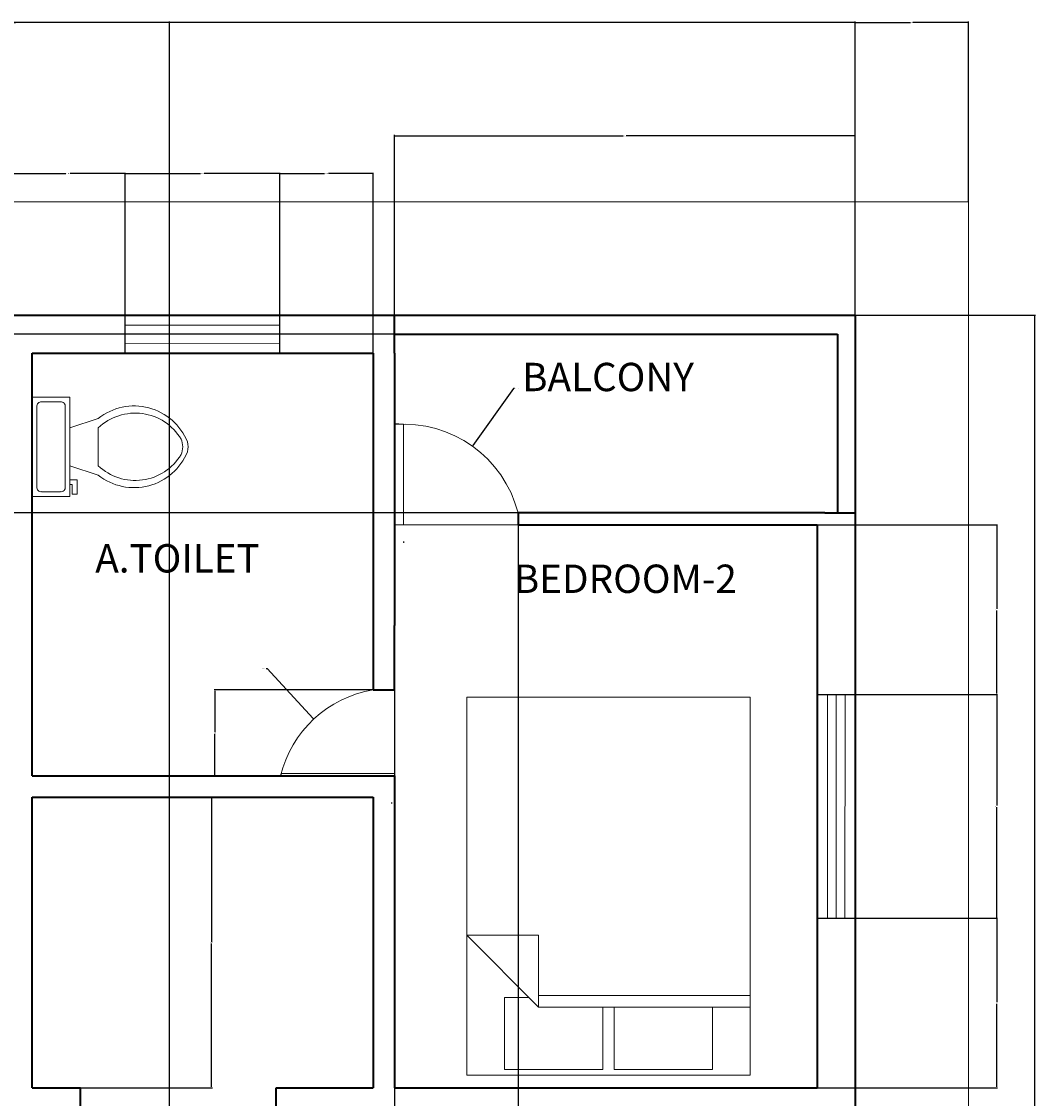
# Model space of a CAD drawing. Units: inches. Extents: x 4700 to 5209, y 8078 to 8754.
# Tile 5 of 5: x 4970 to 5185, y 8526 to 8754. Entities that reach past the tile are written whole.
import ezdxf

# ---------------------------------------------------------------- set-up
doc = ezdxf.new("R2010")
doc.units = ezdxf.units.IN
for name, color, linetype, lineweight in [('A-ANNO-DIMS', 2, 'Continuous', 18), ('A-AREA-IDEN', 7, 'Continuous', 18), ('A-DOOR', 3, 'Continuous', 18), ('A-FLOR-FIXT', 9, 'Continuous', 18), ('A-FURN', 8, 'Continuous', 18), ('A-GLAZ', 4, 'Continuous', 18), ('A-WALL', 7, 'Continuous', 35), ('C-PROP', 8, 'Continuous', 18)]:
    doc.layers.add(name, color=color, linetype=linetype, lineweight=lineweight)
doc.styles.get("Standard").update_dxf_attribs({"font": 'arial.ttf'})
doc.dimstyles.get("Standard").update_dxf_attribs({"dimtxt": 0.18, "dimasz": 0.18, "dimexe": 0.18, "dimexo": 0.0625, "dimgap": 0.09, "dimtad": 0, "dimtih": 1, "dimtoh": 1, "dimdec": 4, "dimzin": 0, "dimdsep": 46, "dimtxsty": 'Standard', "dimcen": 0.09, "dimadec": 0, "dimazin": 0, "dimtfac": 1, "dimtdec": 4, "dimtofl": 0, "dimtmove": 0, "dimatfit": 3, "dimfxl": 1, "dimtolj": 1, "dimtzin": 0, "dimarcsym": 0})

# ---------------------------------------------------------------- blocks, each defined once
blk = doc.blocks.new('Bed - Queen')
for p, q in [((0, -80.00003), (0, 0)), ((0, 0), (59.99999, 0)), ((59.99999, 0), (59.99999, -80.00003)), ((7.99999, -1.2), (28.79998, -1.2)), ((7.99999, -14.4), (7.99999, -1.2)), ((28.79998, -1.2), (28.79998, -14.4)), ((31.19999, -1.2), (51.99999, -1.2)), ((31.19999, -14.4), (31.19999, -1.2)), ((51.99999, -1.2), (51.99999, -16.4)), ((0, -14.4), (44.8, -14.4)), ((59.99999, -29.6), (44.8, -14.4)), ((44.8, -14.4), (44.8, -29.6)), ((44.8, -16.8), (0, -16.8)), ((51.99999, -16.4), (46.79936, -16.4)), ((44.8, -29.6), (59.99999, -29.6)), ((59.99999, -80.00003), (0, -80.00003))]:
    blk.add_line(p, q)
blk = doc.blocks.new('Toilet - top')
for p, q in [((9.5, -6), (9.5, -2)), ((-10, -8.5), (-8, -8.5)), ((-10, -9.5), (-10, -8.5)), ((-8, -8.5), (-8, -8)), ((-7, -8), (-7, -9.5)), ((-4, -8), (-6, -14)), ((4, -8), (6, -14)), ((-7, -9.5), (-10, -9.5)), ((4, -14), (-4, -14))]:
    blk.add_line(p, q)
blk.add_lwpolyline([(10.5, -8), (10.5, 0), (-10.5, 0), (-10.5, -8)], close=True)
for points in [[(-9.5, -2), (-9.5, -6)], [(8.5, -1), (-8.5, -1)], [(-8.5, -7), (8.5, -7)]]:
    blk.add_lwpolyline(points)
for centre, radius, start, end in [((-8.62, -1.88), 0.884, 81.8699, 188.1301), ((8.62, -1.88), 0.884, 351.8699, 98.1301), ((-8.62, -6.12), 0.884, 171.8699, 278.1301), ((8.62, -6.12), 0.884, 261.8699, 8.1301), ((3.52, -21.58), 12.17, 141.4691, 247.9714), ((4.2, -21.82), 11.33, 136.3677, 238.9468), ((-3.52, -21.58), 12.17, 292.0284, 38.5307), ((-4.2, -21.82), 11.33, 301.053, 43.6321), ((0, -27.88), 4, 245.7318, 294.2682), ((0, -29), 4, 254.8605, 285.1395)]:
    blk.add_arc(centre, radius, start, end)
blk = doc.blocks.new('*D16')
at = {"layer": 'A-ANNO-DIMS', "color": 0, "lineweight": -2, "transparency": 16777216}
for p, q in [((4762.78, 8691.81), (4762.78, 8753.93)), ((4762.96, 8753.75), (4954.49, 8753.75)), ((5146.6, 8753.75), (4955.07, 8753.75)), ((5146.78, 8691.81), (5146.78, 8753.93))]:
    blk.add_line(p, q, dxfattribs=at)
at = {"layer": 'A-ANNO-DIMS', "color": 0, "transparency": 16777216}
for points in [[(4762.96, 8753.78), (4762.96, 8753.72), (4762.78, 8753.75)], [(5146.6, 8753.78), (5146.6, 8753.72), (5146.78, 8753.75)]]:
    blk.add_solid(points, dxfattribs=at)
at = {"layer": 'Defpoints', "color": 0, "transparency": 16777216}
for p in [(5146.78, 8753.75), (4762.78, 8691.75), (5146.78, 8691.75)]:
    blk.add_point(p, dxfattribs=at)
at = {"layer": 'A-ANNO-DIMS', "color": 0, "transparency": 16777216, "insert": (4954.78, 8753.75), "char_height": 0.18, "attachment_point": 5}
blk.add_mtext('\\A1;384', dxfattribs=at)
blk = doc.blocks.new('*D17')
at = {"layer": 'A-ANNO-DIMS', "color": 0, "lineweight": -2, "transparency": 16777216}
for p, q in [((5146.84, 8691.75), (5184.96, 8691.75)), ((5184.78, 8691.57), (5184.78, 8403.93)), ((5184.78, 8115.93), (5184.78, 8403.57)), ((5146.84, 8115.75), (5184.96, 8115.75))]:
    blk.add_line(p, q, dxfattribs=at)
at = {"layer": 'A-ANNO-DIMS', "color": 0, "transparency": 16777216}
for points in [[(5184.75, 8691.57), (5184.81, 8691.57), (5184.78, 8691.75)], [(5184.75, 8115.93), (5184.81, 8115.93), (5184.78, 8115.75)]]:
    blk.add_solid(points, dxfattribs=at)
at = {"layer": 'Defpoints', "color": 0, "transparency": 16777216}
for p in [(5146.78, 8691.75), (5146.78, 8115.75), (5184.78, 8115.75)]:
    blk.add_point(p, dxfattribs=at)
at = {"layer": 'A-ANNO-DIMS', "color": 0, "transparency": 16777216, "insert": (5184.78, 8403.75), "char_height": 0.18, "attachment_point": 5}
blk.add_mtext('\\A1;576', dxfattribs=at)
blk = doc.blocks.new('*D24')
at = {"layer": 'A-ANNO-DIMS', "color": 0, "lineweight": -2, "transparency": 16777216}
for p, q in [((4968.07, 8683.81), (4968.07, 8721.93)), ((4968.25, 8721.75), (4979.68, 8721.75)), ((4992.05, 8721.75), (4980.61, 8721.75)), ((4992.23, 8683.81), (4992.23, 8721.93))]:
    blk.add_line(p, q, dxfattribs=at)
at = {"layer": 'A-ANNO-DIMS', "color": 0, "transparency": 16777216}
for points in [[(4968.25, 8721.78), (4968.25, 8721.72), (4968.07, 8721.75)], [(4992.05, 8721.78), (4992.05, 8721.72), (4992.23, 8721.75)]]:
    blk.add_solid(points, dxfattribs=at)
at = {"layer": 'Defpoints', "color": 0, "transparency": 16777216}
for p in [(4992.23, 8721.75), (4968.07, 8683.75), (4992.23, 8683.75)]:
    blk.add_point(p, dxfattribs=at)
at = {"layer": 'A-ANNO-DIMS', "color": 0, "transparency": 16777216, "insert": (4980.15, 8721.75), "char_height": 0.18, "attachment_point": 5}
blk.add_mtext('\\A1;24.153', dxfattribs=at)
blk = doc.blocks.new('*D25')
at = {"layer": 'A-ANNO-DIMS', "color": 0, "lineweight": -2, "transparency": 16777216}
for p, q in [((4992.23, 8683.81), (4992.23, 8721.93)), ((4992.41, 8721.75), (5008.22, 8721.75)), ((5024.82, 8721.75), (5009.01, 8721.75)), ((5025, 8683.81), (5025, 8721.93))]:
    blk.add_line(p, q, dxfattribs=at)
at = {"layer": 'A-ANNO-DIMS', "color": 0, "transparency": 16777216}
for points in [[(4992.41, 8721.78), (4992.41, 8721.72), (4992.23, 8721.75)], [(5024.82, 8721.78), (5024.82, 8721.72), (5025, 8721.75)]]:
    blk.add_solid(points, dxfattribs=at)
at = {"layer": 'Defpoints', "color": 0, "transparency": 16777216}
for p in [(5025, 8721.75), (4992.23, 8683.75), (5025, 8683.75)]:
    blk.add_point(p, dxfattribs=at)
at = {"layer": 'A-ANNO-DIMS', "color": 0, "transparency": 16777216, "insert": (5008.61, 8721.75), "char_height": 0.18, "attachment_point": 5}
blk.add_mtext('\\A1;32.77', dxfattribs=at)
blk = doc.blocks.new('*D26')
at = {"layer": 'A-ANNO-DIMS', "color": 0, "lineweight": -2, "transparency": 16777216}
for p, q in [((5025, 8683.81), (5025, 8721.93)), ((5025.18, 8721.75), (5034.43, 8721.75)), ((5044.6, 8721.75), (5035.34, 8721.75)), ((5044.78, 8683.81), (5044.78, 8721.93))]:
    blk.add_line(p, q, dxfattribs=at)
at = {"layer": 'A-ANNO-DIMS', "color": 0, "transparency": 16777216}
for points in [[(5025.18, 8721.78), (5025.18, 8721.72), (5025, 8721.75)], [(5044.6, 8721.78), (5044.6, 8721.72), (5044.78, 8721.75)]]:
    blk.add_solid(points, dxfattribs=at)
at = {"layer": 'Defpoints', "color": 0, "transparency": 16777216}
for p in [(5044.78, 8721.75), (5025, 8683.75), (5044.78, 8683.75)]:
    blk.add_point(p, dxfattribs=at)
at = {"layer": 'A-ANNO-DIMS', "color": 0, "transparency": 16777216, "insert": (5034.89, 8721.75), "char_height": 0.18, "attachment_point": 5}
blk.add_mtext('\\A1;19.782', dxfattribs=at)
blk = doc.blocks.new('*D27')
at = {"layer": 'A-ANNO-DIMS', "color": 0, "lineweight": -2, "transparency": 16777216}
for p, q in [((5049.28, 8691.81), (5049.28, 8729.93)), ((5049.46, 8729.75), (5097.71, 8729.75)), ((5146.6, 8729.75), (5098.35, 8729.75)), ((5146.78, 8691.81), (5146.78, 8729.93))]:
    blk.add_line(p, q, dxfattribs=at)
at = {"layer": 'A-ANNO-DIMS', "color": 0, "transparency": 16777216}
for points in [[(5049.46, 8729.78), (5049.46, 8729.72), (5049.28, 8729.75)], [(5146.6, 8729.78), (5146.6, 8729.72), (5146.78, 8729.75)]]:
    blk.add_solid(points, dxfattribs=at)
at = {"layer": 'Defpoints', "color": 0, "transparency": 16777216}
for p in [(5146.78, 8729.75), (5049.28, 8691.75), (5146.78, 8691.75)]:
    blk.add_point(p, dxfattribs=at)
at = {"layer": 'A-ANNO-DIMS', "color": 0, "transparency": 16777216, "insert": (5098.03, 8729.75), "char_height": 0.18, "attachment_point": 5}
blk.add_mtext('\\A1;97.5', dxfattribs=at)
blk = doc.blocks.new('*D44')
at = {"layer": 'A-ANNO-DIMS', "color": 0, "lineweight": -2, "transparency": 16777216}
for p, q in [((5138.84, 8564.15), (5176.96, 8564.15)), ((5176.78, 8563.97), (5176.78, 8546.38)), ((5176.78, 8528.43), (5176.78, 8546.02)), ((5138.84, 8528.25), (5176.96, 8528.25))]:
    blk.add_line(p, q, dxfattribs=at)
at = {"layer": 'A-ANNO-DIMS', "color": 0, "transparency": 16777216}
for points in [[(5176.75, 8563.97), (5176.81, 8563.97), (5176.78, 8564.15)], [(5176.75, 8528.43), (5176.81, 8528.43), (5176.78, 8528.25)]]:
    blk.add_solid(points, dxfattribs=at)
at = {"layer": 'Defpoints', "color": 0, "transparency": 16777216}
for p in [(5138.78, 8564.15), (5138.78, 8528.25), (5176.78, 8528.25)]:
    blk.add_point(p, dxfattribs=at)
at = {"layer": 'A-ANNO-DIMS', "color": 0, "transparency": 16777216, "insert": (5176.78, 8546.2), "char_height": 0.18, "attachment_point": 5}
blk.add_mtext('\\A1;35.9', dxfattribs=at)
blk = doc.blocks.new('*D45')
at = {"layer": 'A-ANNO-DIMS', "color": 0, "lineweight": -2, "transparency": 16777216}
for p, q in [((5138.84, 8611.51), (5176.96, 8611.51)), ((5176.78, 8611.33), (5176.78, 8588.01)), ((5176.78, 8564.33), (5176.78, 8587.65)), ((5138.84, 8564.15), (5176.96, 8564.15))]:
    blk.add_line(p, q, dxfattribs=at)
at = {"layer": 'A-ANNO-DIMS', "color": 0, "transparency": 16777216}
for points in [[(5176.75, 8611.33), (5176.81, 8611.33), (5176.78, 8611.51)], [(5176.75, 8564.33), (5176.81, 8564.33), (5176.78, 8564.15)]]:
    blk.add_solid(points, dxfattribs=at)
at = {"layer": 'Defpoints', "color": 0, "transparency": 16777216}
for p in [(5138.78, 8611.51), (5138.78, 8564.15), (5176.78, 8564.15)]:
    blk.add_point(p, dxfattribs=at)
at = {"layer": 'A-ANNO-DIMS', "color": 0, "transparency": 16777216, "insert": (5176.78, 8587.83), "char_height": 0.18, "attachment_point": 5}
blk.add_mtext('\\A1;47.36', dxfattribs=at)
blk = doc.blocks.new('*D46')
at = {"layer": 'A-ANNO-DIMS', "color": 0, "lineweight": -2, "transparency": 16777216}
for p, q in [((5138.84, 8647.41), (5176.96, 8647.41)), ((5176.78, 8647.23), (5176.78, 8629.64)), ((5176.78, 8611.69), (5176.78, 8629.28)), ((5138.84, 8611.51), (5176.96, 8611.51))]:
    blk.add_line(p, q, dxfattribs=at)
at = {"layer": 'A-ANNO-DIMS', "color": 0, "transparency": 16777216}
for points in [[(5176.75, 8647.23), (5176.81, 8647.23), (5176.78, 8647.41)], [(5176.75, 8611.69), (5176.81, 8611.69), (5176.78, 8611.51)]]:
    blk.add_solid(points, dxfattribs=at)
at = {"layer": 'Defpoints', "color": 0, "transparency": 16777216}
for p in [(5138.78, 8647.41), (5138.78, 8611.51), (5176.78, 8611.51)]:
    blk.add_point(p, dxfattribs=at)
at = {"layer": 'A-ANNO-DIMS', "color": 0, "transparency": 16777216, "insert": (5176.78, 8629.46), "char_height": 0.18, "attachment_point": 5}
blk.add_mtext('\\A1;35.89', dxfattribs=at)
blk = doc.blocks.new('*D47')
at = {"layer": 'A-ANNO-DIMS', "color": 0, "lineweight": -2, "transparency": 16777216}
for p, q in [((5142.99, 8687.75), (4700.6, 8687.75)), ((4700.78, 8687.57), (4700.78, 8669.03)), ((4700.78, 8650.12), (4700.78, 8668.66)), ((5142.99, 8649.94), (4700.6, 8649.94))]:
    blk.add_line(p, q, dxfattribs=at)
at = {"layer": 'A-ANNO-DIMS', "color": 0, "transparency": 16777216}
for points in [[(4700.75, 8687.57), (4700.81, 8687.57), (4700.78, 8687.75)], [(4700.75, 8650.12), (4700.81, 8650.12), (4700.78, 8649.94)]]:
    blk.add_solid(points, dxfattribs=at)
at = {"layer": 'Defpoints', "color": 0, "transparency": 16777216}
for p in [(5143.05, 8687.75), (4700.78, 8649.94), (5143.05, 8649.94)]:
    blk.add_point(p, dxfattribs=at)
at = {"layer": 'A-ANNO-DIMS', "color": 0, "transparency": 16777216, "insert": (4700.78, 8668.84), "char_height": 0.18, "attachment_point": 5}
blk.add_mtext('\\A1;37.814', dxfattribs=at)
blk = doc.blocks.new('*D55')
at = {"layer": 'A-ANNO-DIMS', "color": 0, "lineweight": -2, "transparency": 16777216}
for p, q in [((4937.15, 8207.81), (4937.15, 8753.93)), ((4937.33, 8753.75), (4969.02, 8753.75)), ((5001.49, 8753.75), (4969.8, 8753.75)), ((5001.67, 8207.81), (5001.67, 8753.93))]:
    blk.add_line(p, q, dxfattribs=at)
at = {"layer": 'A-ANNO-DIMS', "color": 0, "transparency": 16777216}
for points in [[(4937.33, 8753.78), (4937.33, 8753.72), (4937.15, 8753.75)], [(5001.49, 8753.78), (5001.49, 8753.72), (5001.67, 8753.75)]]:
    blk.add_solid(points, dxfattribs=at)
at = {"layer": 'Defpoints', "color": 0, "transparency": 16777216}
for p in [(5001.67, 8753.75), (4937.15, 8207.75), (5001.67, 8207.75)]:
    blk.add_point(p, dxfattribs=at)
at = {"layer": 'A-ANNO-DIMS', "color": 0, "transparency": 16777216, "insert": (4969.41, 8753.75), "char_height": 0.18, "attachment_point": 5}
blk.add_mtext('\\A1;64.53', dxfattribs=at)
blk = doc.blocks.new('*D59')
at = {"layer": 'A-ANNO-DIMS', "color": 0, "lineweight": -2, "transparency": 16777216}
for p, q in [((4972.64, 8589.75), (5010.75, 8589.75)), ((5010.57, 8589.57), (5010.57, 8559.18)), ((5010.57, 8528.43), (5010.57, 8558.82)), ((4972.64, 8528.25), (5010.75, 8528.25))]:
    blk.add_line(p, q, dxfattribs=at)
at = {"layer": 'A-ANNO-DIMS', "color": 0, "transparency": 16777216}
for points in [[(5010.54, 8589.57), (5010.6, 8589.57), (5010.57, 8589.75)], [(5010.54, 8528.43), (5010.6, 8528.43), (5010.57, 8528.25)]]:
    blk.add_solid(points, dxfattribs=at)
at = {"layer": 'Defpoints', "color": 0, "transparency": 16777216}
for p in [(4972.57, 8589.75), (4972.57, 8528.25), (5010.57, 8528.25)]:
    blk.add_point(p, dxfattribs=at)
at = {"layer": 'A-ANNO-DIMS', "color": 0, "transparency": 16777216, "insert": (5010.57, 8559), "char_height": 0.18, "attachment_point": 5}
blk.add_mtext('\\A1;61.5', dxfattribs=at)
blk = doc.blocks.new('*D68')
at = {"layer": 'A-ANNO-DIMS', "color": 0, "lineweight": -2, "transparency": 16777216}
for p, q in [((5049.22, 8612.47), (5011.1, 8612.47)), ((5011.28, 8612.29), (5011.28, 8603.54)), ((5011.28, 8594.43), (5011.28, 8603.18)), ((5049.22, 8594.25), (5011.1, 8594.25))]:
    blk.add_line(p, q, dxfattribs=at)
at = {"layer": 'A-ANNO-DIMS', "color": 0, "transparency": 16777216}
for points in [[(5011.25, 8612.29), (5011.31, 8612.29), (5011.28, 8612.47)], [(5011.25, 8594.43), (5011.31, 8594.43), (5011.28, 8594.25)]]:
    blk.add_solid(points, dxfattribs=at)
at = {"layer": 'Defpoints', "color": 0, "transparency": 16777216}
for p in [(5011.28, 8612.47), (5049.28, 8612.47), (5049.28, 8594.25)]:
    blk.add_point(p, dxfattribs=at)
at = {"layer": 'A-ANNO-DIMS', "color": 0, "transparency": 16777216, "insert": (5011.28, 8603.36), "char_height": 0.18, "attachment_point": 5}
blk.add_mtext('\\A1;18.215', dxfattribs=at)
blk = doc.blocks.new('*D71')
at = {"layer": 'A-ANNO-DIMS', "color": 0, "lineweight": -2, "transparency": 16777216}
for p, q in [((5049.28, 8647.34), (5049.28, 8077.57)), ((5075.44, 8647.34), (5075.44, 8077.57)), ((5049.46, 8077.75), (5061.97, 8077.75)), ((5075.26, 8077.75), (5062.76, 8077.75))]:
    blk.add_line(p, q, dxfattribs=at)
at = {"layer": 'A-ANNO-DIMS', "color": 0, "transparency": 16777216}
for points in [[(5049.46, 8077.78), (5049.46, 8077.72), (5049.28, 8077.75)], [(5075.26, 8077.78), (5075.26, 8077.72), (5075.44, 8077.75)]]:
    blk.add_solid(points, dxfattribs=at)
at = {"layer": 'Defpoints', "color": 0, "transparency": 16777216}
for p in [(5049.28, 8647.41), (5075.44, 8647.41), (5075.44, 8077.75)]:
    blk.add_point(p, dxfattribs=at)
at = {"layer": 'A-ANNO-DIMS', "color": 0, "transparency": 16777216, "insert": (5062.36, 8077.75), "char_height": 0.18, "attachment_point": 5}
blk.add_mtext('\\A1;26.16', dxfattribs=at)
blk = doc.blocks.new('*D73')
at = {"layer": 'A-ANNO-DIMS', "color": 0, "lineweight": -2, "transparency": 16777216}
for p, q in [((5146.78, 8691.81), (5146.78, 8753.93)), ((5146.96, 8753.75), (5158.56, 8753.75)), ((5170.6, 8753.75), (5159, 8753.75)), ((5170.78, 8715.81), (5170.78, 8753.93))]:
    blk.add_line(p, q, dxfattribs=at)
at = {"layer": 'A-ANNO-DIMS', "color": 0, "transparency": 16777216}
for points in [[(5146.96, 8753.78), (5146.96, 8753.72), (5146.78, 8753.75)], [(5170.6, 8753.78), (5170.6, 8753.72), (5170.78, 8753.75)]]:
    blk.add_solid(points, dxfattribs=at)
at = {"layer": 'Defpoints', "color": 0, "transparency": 16777216}
for p in [(5170.78, 8753.75), (5170.78, 8715.75), (5146.78, 8691.75)]:
    blk.add_point(p, dxfattribs=at)
at = {"layer": 'A-ANNO-DIMS', "color": 0, "transparency": 16777216, "insert": (5158.78, 8753.75), "char_height": 0.18, "attachment_point": 5}
blk.add_mtext('\\A1;24', dxfattribs=at)
blk = doc.blocks.new('*D83')
at = {"layer": 'A-ANNO-DIMS', "color": 0, "lineweight": -2, "transparency": 16777216}
for p, q in [((5074.48, 8676.24), (5065.88, 8664.21)), ((5074.66, 8676.24), (5074.48, 8676.24)), ((5051.17, 8643.76), (5051.35, 8643.76)), ((5051.26, 8643.67), (5051.26, 8643.85))]:
    blk.add_line(p, q, dxfattribs=at)
at = {"layer": 'A-ANNO-DIMS', "color": 0, "transparency": 16777216}
blk.add_solid([(5065.85, 8664.23), (5065.9, 8664.19), (5065.77, 8664.06)], dxfattribs=at)
at = {"layer": 'Defpoints', "color": 0, "transparency": 16777216}
for p in [(5065.77, 8664.06), (5051.26, 8643.76)]:
    blk.add_point(p, dxfattribs=at)
at = {"layer": 'A-ANNO-DIMS', "color": 0, "transparency": 16777216, "insert": (5075.21, 8676.24), "char_height": 0.18, "attachment_point": 5}
blk.add_mtext('\\A1;R24.955', dxfattribs=at)
blk = doc.blocks.new('*D84')
at = {"layer": 'A-ANNO-DIMS', "color": 0, "lineweight": -2, "transparency": 16777216}
for p, q in [((5022.15, 8616.98), (5022.33, 8616.98)), ((5022.33, 8616.98), (5032.09, 8606.45)), ((5048.6, 8588.55), (5048.78, 8588.55)), ((5048.69, 8588.46), (5048.69, 8588.64))]:
    blk.add_line(p, q, dxfattribs=at)
at = {"layer": 'A-ANNO-DIMS', "color": 0, "transparency": 16777216}
blk.add_solid([(5032.11, 8606.47), (5032.07, 8606.43), (5032.21, 8606.32)], dxfattribs=at)
at = {"layer": 'Defpoints', "color": 0, "transparency": 16777216}
for p in [(5032.21, 8606.32), (5048.69, 8588.55)]:
    blk.add_point(p, dxfattribs=at)
at = {"layer": 'A-ANNO-DIMS', "color": 0, "transparency": 16777216, "insert": (5021.67, 8616.98), "char_height": 0.18, "attachment_point": 5}
blk.add_mtext('\\A1;R24.23', dxfattribs=at)

msp = doc.modelspace()

# ---------------------------------------------------------------- linework, layer by layer
at = {"layer": 'A-DOOR'}
for p, q in [((5051.21, 8668.7155), (5049.2803, 8668.8641)), ((5051.21, 8647.4059), (5051.21, 8668.7155)), ((5049.2803, 8647.4059), (5051.21, 8647.4059)), ((5051.21, 8647.4059), (5075.4408, 8647.4059)), ((5049.2803, 8612.4657), (5049.2803, 8594.2503)), ((5049.2803, 8594.7861), (5025.2753, 8594.7861)), ((5025.2753, 8594.7861), (5025.2753, 8594.2503)), ((5049.2803, 8594.2503), (5049.2803, 8594.7861))]:
    msp.add_line(p, q, dxfattribs=at)
for centre, radius, start, end in [((5051.2623, 8643.7608), 24.9547, 14.328007, 94.555505), ((5048.6891, 8588.5541), 24.229, 99.28391, 166.402517)]:
    msp.add_arc(centre, radius, start, end, dxfattribs=at)
at = {"layer": 'A-GLAZ'}
for p, q in [((4992.2261, 8689.6376), (5024.9979, 8689.6376)), ((4992.2261, 8687.7503), (5024.9979, 8687.7503)), ((4992.2261, 8685.876), (5024.9979, 8685.8133)), ((5140.9607, 8611.5136), (5140.9607, 8564.1518)), ((5142.7803, 8611.5136), (5142.7803, 8564.1518)), ((5144.7087, 8611.5136), (5144.6194, 8564.1518))]:
    msp.add_line(p, q, dxfattribs=at)
for points in [[(4992.2261, 8691.7503), (5024.9979, 8691.7503), (5024.9979, 8683.7503), (4992.2261, 8683.7503)], [(5138.7803, 8611.5136), (5146.7803, 8611.5136), (5146.7803, 8564.1518), (5138.7803, 8564.1518)]]:
    msp.add_lwpolyline(points, close=True, dxfattribs=at)
at = {"layer": 'A-WALL'}
for p, q in [((4762.7803, 8691.7503), (5146.7803, 8691.7503)), ((5049.2803, 8683.7503), (5049.2803, 8691.7503)), ((5146.7803, 8691.7503), (5146.7803, 8199.7503)), ((5049.2803, 8687.7503), (5143.0547, 8687.7503)), ((5143.0547, 8687.7503), (5143.0547, 8649.9364)), ((4972.5733, 8683.7503), (5044.7803, 8683.7503)), ((4972.5733, 8594.2503), (4972.5733, 8683.7503)), ((5044.7803, 8683.7503), (5044.7803, 8626.0977)), ((5049.2803, 8683.7503), (5049.2803, 8626.0977)), ((5140.3862, 8649.9364), (5075.4408, 8649.9364)), ((5075.4408, 8649.9364), (5075.4408, 8647.4059)), ((5140.3862, 8649.9364), (5146.7803, 8649.9364)), ((5075.4408, 8647.4059), (5138.7803, 8647.4059)), ((5138.7803, 8647.4059), (5138.7803, 8528.2503)), ((5044.7803, 8626.0977), (5044.7803, 8612.4657)), ((5049.2803, 8612.4657), (5049.2803, 8626.0977)), ((5044.7803, 8612.4657), (5049.2803, 8612.4657)), ((4972.5733, 8594.2503), (5044.7803, 8594.2503)), ((5044.7803, 8594.2503), (5049.2803, 8594.2503)), ((5049.2803, 8594.2503), (5049.2803, 8528.2503)), ((4972.5733, 8528.2503), (4972.5733, 8589.7503)), ((4972.5733, 8589.7503), (5044.7803, 8589.7503)), ((5044.7803, 8589.7503), (5044.7803, 8528.2503)), ((4972.5733, 8528.2503), (4982.778, 8528.2503)), ((4982.778, 8523.7503), (4982.778, 8528.2503)), ((5024.2192, 8523.7503), (5024.2192, 8528.2503)), ((5024.2192, 8528.2503), (5044.7803, 8528.2503)), ((5049.2803, 8528.2503), (5138.7803, 8528.2503))]:
    msp.add_line(p, q, dxfattribs=at)
at = {"layer": 'C-PROP'}
for p, q in [((4738.7803, 8715.7503), (5170.7803, 8715.7503)), ((5170.7803, 8715.7503), (5170.7803, 8115.7503))]:
    msp.add_line(p, q, dxfattribs=at)

# ---------------------------------------------------------------- block references
at = {"layer": 'A-FLOR-FIXT', "rotation": 90}
msp.add_blockref('Toilet - top', (4972.5733, 8663.9273), dxfattribs=at)
at = {"layer": 'A-FURN', "rotation": 180}
msp.add_blockref('Bed - Queen', (5124.601, 8530.9577), dxfattribs=at)

# ---------------------------------------------------------------- texts
at = {"layer": 'A-AREA-IDEN', "char_height": 6, "attachment_point": 1}
for s, insert in [('\\pxi-3,l4,t4;BALCONY ', (5070.3103, 8681.6976)), ('\\pxi-3,l4,t4;A.TOILET', (4979.9369, 8643.3167)), ('\\pxi-3,l4,t4;BEDROOM-2', (5068.5498, 8638.9918))]:
    msp.add_mtext_dynamic_manual_height_columns(s, width=51.756341, gutter_width=12.5, heights=[0], dxfattribs=dict(at, insert=insert))

# ---------------------------------------------------------------- dimensions: what is measured, and where the dimension line sits
at = {"layer": 'A-ANNO-DIMS'}
for base, p1, p2, override, picture, middle in [((5146.7803, 8753.7503), (4762.7803, 8691.7503), (5146.7803, 8691.7503), {"dimdec": 0, "dimlfac": 1, "dimrnd": 0, "dimzin": 0, "dimdsep": 46, "dimlunit": 2}, '*D16', (4954.7803, 8753.7503)), ((5001.6744, 8753.7503), (4937.1464, 8207.7503), (5001.6744, 8207.7503), {"dimdec": 2, "dimlfac": 1, "dimrnd": 0, "dimzin": 0, "dimdsep": 46, "dimlunit": 2}, '*D55', (4969.4104, 8753.7503)), ((5170.7803, 8753.7503), (5146.7803, 8691.7503), (5170.7803, 8715.7503), {"dimdec": 0, "dimlfac": 1, "dimrnd": 0, "dimzin": 0, "dimdsep": 46, "dimlunit": 2}, '*D73', (5158.7803, 8753.7503)), ((5146.7803, 8729.7503), (5049.2803, 8691.7503), (5146.7803, 8691.7503), {"dimdec": 1, "dimlfac": 1, "dimrnd": 0, "dimzin": 0, "dimdsep": 46, "dimlunit": 2}, '*D27', (5098.0303, 8729.7503)), ((4992.2261, 8721.7503), (4968.0733, 8683.7503), (4992.2261, 8683.7503), {"dimdec": 3, "dimlfac": 1, "dimrnd": 0, "dimzin": 0, "dimdsep": 46, "dimlunit": 2}, '*D24', (4980.1497, 8721.7503)), ((5024.9979, 8721.7503), (4992.2261, 8683.7503), (5024.9979, 8683.7503), {"dimdec": 2, "dimlfac": 1, "dimrnd": 0, "dimzin": 0, "dimdsep": 46, "dimlunit": 2}, '*D25', (5008.612, 8721.7503)), ((5044.7803, 8721.7503), (5024.9979, 8683.7503), (5044.7803, 8683.7503), {"dimdec": 3, "dimlfac": 1, "dimrnd": 0, "dimzin": 0, "dimdsep": 46, "dimlunit": 2}, '*D26', (5034.8891, 8721.7503)), ((5075.4408, 8077.7503), (5049.2803, 8647.4059), (5075.4408, 8647.4059), {"dimdec": 2, "dimlfac": 1, "dimrnd": 0, "dimzin": 0, "dimdsep": 46, "dimlunit": 2}, '*D71', (5062.3606, 8077.7503))]:
    dim = msp.add_linear_dim(base=base, p1=p1, p2=p2, dimstyle='Standard', override=override, dxfattribs=at)
    dim.commit()
    dim.dimension.update_dxf_attribs({"geometry": picture, "text_midpoint": middle})
for base, p1, p2, angle, override, picture, middle in [((5184.7803, 8115.7503), (5146.7803, 8691.7503), (5146.7803, 8115.7503), 270, {"dimdec": 0, "dimlfac": 1, "dimrnd": 0, "dimzin": 0, "dimdsep": 46, "dimlunit": 2}, '*D17', (5184.7803, 8403.7503)), ((4700.7803, 8649.9364), (5143.0547, 8687.7503), (5143.0547, 8649.9364), 90, {"dimdec": 3, "dimlfac": 1, "dimrnd": 0, "dimzin": 0, "dimdsep": 46, "dimlunit": 2}, '*D47', (4700.7803, 8668.8434)), ((5176.7803, 8611.5136), (5138.7803, 8647.4059), (5138.7803, 8611.5136), 270, {"dimdec": 2, "dimlfac": 1, "dimrnd": 0, "dimzin": 0, "dimdsep": 46, "dimlunit": 2}, '*D46', (5176.7803, 8629.4597)), ((5011.2803, 8612.4657), (5049.2803, 8594.2503), (5049.2803, 8612.4657), 90, {"dimdec": 3, "dimlfac": 1, "dimrnd": 0, "dimzin": 0, "dimdsep": 46, "dimlunit": 2}, '*D68', (5011.2803, 8603.358)), ((5176.7803, 8564.1518), (5138.7803, 8611.5136), (5138.7803, 8564.1518), 270, {"dimdec": 2, "dimlfac": 1, "dimrnd": 0, "dimzin": 0, "dimdsep": 46, "dimlunit": 2}, '*D45', (5176.7803, 8587.8327)), ((5010.5733, 8528.2503), (4972.5733, 8589.7503), (4972.5733, 8528.2503), 270, {"dimdec": 1, "dimlfac": 1, "dimrnd": 0, "dimzin": 0, "dimdsep": 46, "dimlunit": 2}, '*D59', (5010.5733, 8559.0003)), ((5176.7803, 8528.2503), (5138.7803, 8564.1518), (5138.7803, 8528.2503), 270, {"dimdec": 1, "dimlfac": 1, "dimrnd": 0, "dimzin": 0, "dimdsep": 46, "dimlunit": 2}, '*D44', (5176.7803, 8546.201))]:
    dim = msp.add_linear_dim(base=base, p1=p1, p2=p2, angle=angle, dimstyle='Standard', override=override, dxfattribs=at)
    dim.commit()
    dim.dimension.update_dxf_attribs({"geometry": picture, "text_midpoint": middle})
for center, mpoint, override, picture, middle in [((5051.2623, 8643.7608), (5065.7741, 8664.0622), {"dimdec": 3, "dimlfac": 1, "dimrnd": 0, "dimzin": 0, "dimdsep": 46, "dimlunit": 2}, '*D83', (5075.2117, 8676.243)), ((5048.6891, 8588.5541), (5032.2137, 8606.3194), {"dimdec": 2, "dimlfac": 1, "dimrnd": 0, "dimzin": 0, "dimdsep": 46, "dimlunit": 2}, '*D84', (5021.6686, 8616.9785))]:
    dim = msp.add_radius_dim(center=center, mpoint=mpoint, dimstyle='Standard', override=override, dxfattribs=at)
    dim.commit()
    dim.dimension.update_dxf_attribs({"geometry": picture, "text_midpoint": middle, "dimtype": 164})

doc.saveas('drawing.dxf')
